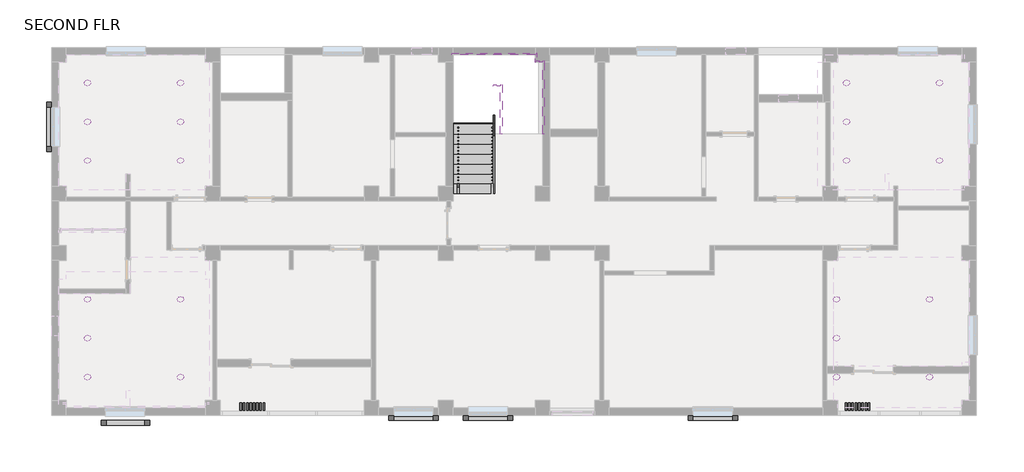
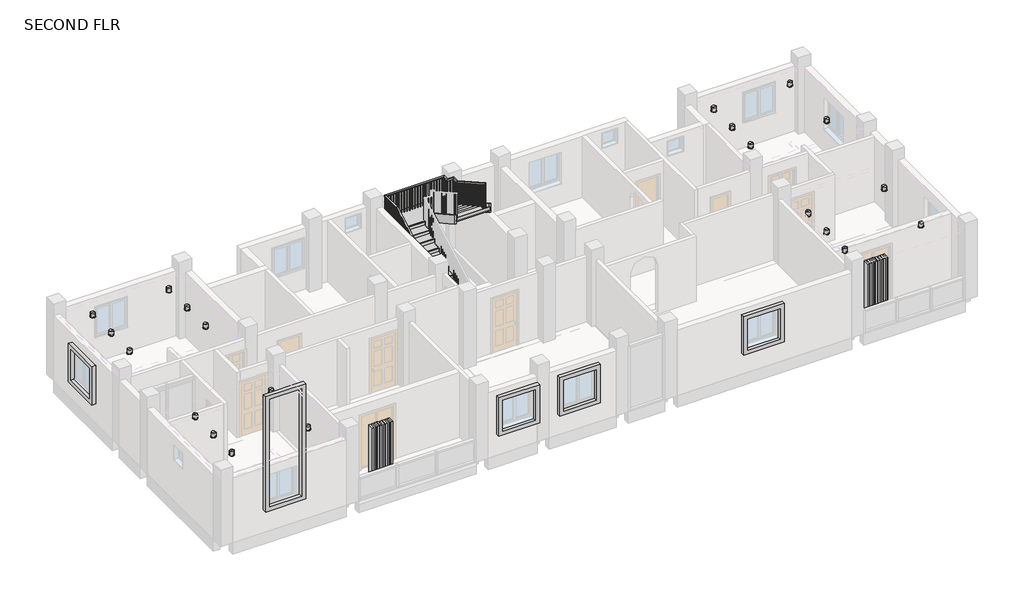
# One storey, part 5 of 5: 21 light fixtures, 8 members, 7 proxies, 1 railing, 1 stair flight.
# Revit data of these elements (continued)
# Elements 29, 30, 31, 32, 33, 34, 35, 36 (IfcMember, "Stringer - 2\" Width")
#   Phase Created = New Construction
# Element 37 (IfcRailing, "Handrail - Rectangular")
#   Phase Created = New Construction
# Element 38 (IfcStairFlight, "2\" Tread 1\" Nosing 1/4\" Riser")
#   Phase Created = New Construction
# Materials
#   "Metal - Paint Finish - Ivory,Glossy": colour RGB 247 247 239, transparency 0
#   "TEAK BROWN COLOUR": class "Generic", colour RGB 120 120 120, transparency 0, Cost = 0
#   "WALL ACCENT 6\"": class "Generic", colour RGB 120 120 120, transparency 0, Cost = 0
